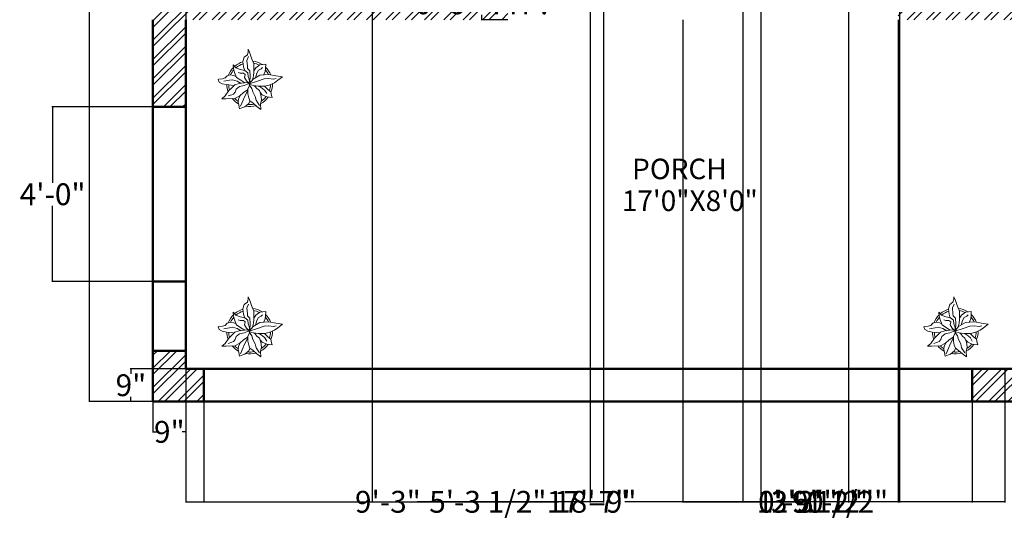
# Model space of a CAD drawing. Units: inches. Extents: x -71 to 434, y -519 to 67.
# Tile 1 of 7: x -49 to 221, y -519 to -377. Entities that reach past the tile are written whole.
import ezdxf

# ---------------------------------------------------------------- set-up
doc = ezdxf.new("R2010")
doc.units = ezdxf.units.IN
doc.header["$MEASUREMENT"] = 0
for name, color, linetype, lineweight in [('A-ANNO-DIMS', 7, 'Continuous', 18), ('A-AREA-IDEN', 7, 'Continuous', 25), ('A-WALL-PATT', 8, 'Continuous', 13), ('CAY', 94, 'Continuous', 13), ('WALL', 50, 'Continuous', 50)]:
    doc.layers.add(name, color=color, linetype=linetype, lineweight=lineweight)
doc.styles.add('ATT', font='romans.shx')
doc.styles.get("Standard").update_dxf_attribs({"font": 'arial.ttf'})
doc.dimstyles.get("Standard").update_dxf_attribs({"dimtxt": 6, "dimasz": 0.18, "dimexe": 0.18, "dimexo": 0.0625, "dimgap": 0.09, "dimtad": 0, "dimtih": 1, "dimtoh": 1, "dimdec": 0, "dimzin": 0, "dimdsep": 46, "dimlunit": 3, "dimtxsty": 'Standard', "dimcen": 0.09, "dimadec": 0, "dimazin": 0, "dimtfac": 1, "dimtdec": 0, "dimtofl": 0, "dimtmove": 0, "dimatfit": 3, "dimfxl": 1, "dimtolj": 1, "dimtzin": 0, "dimarcsym": 0})

# ---------------------------------------------------------------- blocks, each defined once
blk = doc.blocks.new('*D18')
at = {"layer": 'A-ANNO-DIMS', "color": 0, "lineweight": -2, "transparency": 16777216}
for p, q in [((-12.65, 30.83), (-30.15, 30.83)), ((-29.97, 30.65), (-29.97, -222.51)), ((-29.97, -481.99), (-29.97, -228.82)), ((-12.65, -482.17), (-30.15, -482.17))]:
    blk.add_line(p, q, dxfattribs=at)
at = {"layer": 'A-ANNO-DIMS', "color": 0, "transparency": 16777216}
for points in [[(-30, 30.65), (-29.94, 30.65), (-29.97, 30.83)], [(-30, -481.99), (-29.94, -481.99), (-29.97, -482.17)]]:
    blk.add_solid(points, dxfattribs=at)
at = {"layer": 'Defpoints', "color": 0, "transparency": 16777216}
for p in [(-12.59, 30.83), (-29.97, -482.17), (-12.59, -482.17)]:
    blk.add_point(p, dxfattribs=at)
at = {"layer": 'A-ANNO-DIMS', "color": 0, "transparency": 16777216, "insert": (-29.97, -225.67), "char_height": 6, "attachment_point": 5}
blk.add_mtext('\\A1;42\'-9"', dxfattribs=at)
blk = doc.blocks.new('*D19')
at = {"layer": 'A-ANNO-DIMS', "color": 0, "lineweight": -2, "transparency": 16777216}
for p, q in [((-3.65, -473.17), (-18.81, -473.17)), ((-18.63, -473.35), (-18.63, -474.51)), ((-18.63, -481.99), (-18.63, -480.82)), ((-3.65, -482.17), (-18.81, -482.17))]:
    blk.add_line(p, q, dxfattribs=at)
at = {"layer": 'A-ANNO-DIMS', "color": 0, "transparency": 16777216}
for points in [[(-18.66, -473.35), (-18.6, -473.35), (-18.63, -473.17)], [(-18.66, -481.99), (-18.6, -481.99), (-18.63, -482.17)]]:
    blk.add_solid(points, dxfattribs=at)
at = {"layer": 'Defpoints', "color": 0, "transparency": 16777216}
for p in [(-3.59, -473.17), (-18.63, -482.17), (-3.59, -482.17)]:
    blk.add_point(p, dxfattribs=at)
at = {"layer": 'A-ANNO-DIMS', "color": 0, "transparency": 16777216, "insert": (-18.63, -477.67), "char_height": 6, "attachment_point": 5}
blk.add_mtext('\\A1;9"', dxfattribs=at)
blk = doc.blocks.new('*D20')
at = {"layer": 'A-ANNO-DIMS', "color": 0, "lineweight": -2, "transparency": 16777216}
for p, q in [((-12.59, -473.23), (-12.59, -490.67)), ((-3.59, -473.23), (-3.59, -490.67)), ((-12.41, -490.49), (-11.63, -490.49)), ((-3.77, -490.49), (-4.55, -490.49))]:
    blk.add_line(p, q, dxfattribs=at)
at = {"layer": 'A-ANNO-DIMS', "color": 0, "transparency": 16777216}
for points in [[(-12.41, -490.46), (-12.41, -490.52), (-12.59, -490.49)], [(-3.77, -490.46), (-3.77, -490.52), (-3.59, -490.49)]]:
    blk.add_solid(points, dxfattribs=at)
at = {"layer": 'Defpoints', "color": 0, "transparency": 16777216}
for p in [(-12.59, -473.17), (-3.59, -473.17), (-3.59, -490.49)]:
    blk.add_point(p, dxfattribs=at)
at = {"layer": 'A-ANNO-DIMS', "color": 0, "transparency": 16777216, "insert": (-8.09, -490.49), "char_height": 6, "attachment_point": 5}
blk.add_mtext('\\A1;9"', dxfattribs=at)
blk = doc.blocks.new('12PPLT12')
at = {"color": 0, "linetype": 'ByBlock'}
for p, q in [((-0.05, 0.632), (-0.034, 0.694)), ((-0.034, 0.694), (-0.032, 0.751)), ((-0.032, 0.751), (-0.002, 0.689)), ((-0.002, 0.689), (0.044, 0.559)), ((-0.148, 0.486), (-0.116, 0.583)), ((-0.132, 0.367), (-0.148, 0.486)), ((-0.116, 0.583), (-0.05, 0.632)), ((-0.064, 0.51), (-0.026, 0.591)), ((-0.05, 0.38), (-0.064, 0.51)), ((0.044, 0.559), (0.09, 0.432)), ((0.09, 0.432), (0.09, 0.339)), ((-0.349, 0.334), (-0.362, 0.415)), ((-0.362, 0.415), (-0.303, 0.35)), ((-0.332, 0.247), (-0.349, 0.334)), ((-0.289, 0.136), (-0.332, 0.247)), ((-0.303, 0.35), (-0.208, 0.312)), ((-0.205, 0.231), (-0.251, 0.247)), ((-0.208, 0.312), (-0.105, 0.29)), ((-0.137, 0.231), (-0.205, 0.231)), ((-0.097, 0.204), (-0.137, 0.231)), ((-0.108, 0.279), (-0.132, 0.367)), ((-0.105, 0.29), (-0.037, 0.236)), ((-0.043, 0.334), (-0.05, 0.38)), ((0.003, 0.279), (-0.043, 0.334)), ((-0.037, 0.236), (-0.034, 0.158)), ((0.009, 0.169), (0.003, 0.279)), ((0.09, 0.253), (0.082, 0.174)), ((0.09, 0.339), (0.09, 0.253)), ((0.093, 0.282), (0.134, 0.347)), ((0.155, 0.228), (0.131, 0.13)), ((0.134, 0.347), (0.22, 0.415)), ((0.193, 0.293), (0.155, 0.228)), ((0.25, 0.328), (0.193, 0.293)), ((0.22, 0.415), (0.291, 0.421)), ((0.28, 0.353), (0.25, 0.328)), ((0.291, 0.421), (0.35, 0.429)), ((0.342, 0.266), (0.304, 0.19)), ((0.348, 0.331), (0.342, 0.266)), ((0.35, 0.429), (0.348, 0.331)), ((-0.671, 0.098), (-0.687, 0.095)), ((-0.687, 0.095), (-0.666, 0.036)), ((-0.59, 0.109), (-0.671, 0.098)), ((-0.666, 0.036), (-0.601, -0.005)), ((-0.536, 0.125), (-0.59, 0.109)), ((-0.563, 0.052), (-0.441, 0.074)), ((-0.487, 0.171), (-0.536, 0.125)), ((-0.425, 0.193), (-0.487, 0.171)), ((-0.441, 0.074), (-0.373, 0.084)), ((-0.346, 0.179), (-0.425, 0.193)), ((-0.373, 0.084), (-0.27, 0.057)), ((-0.292, 0.149), (-0.346, 0.179)), ((-0.229, 0.003), (-0.324, -0.027)), ((-0.194, 0.074), (-0.289, 0.136)), ((-0.27, 0.057), (-0.186, 0.006)), ((-0.069, 0.027), (-0.229, 0.003)), ((-0.108, 0.019), (-0.194, 0.074)), ((-0.01, 0.003), (-0.121, -0.038)), ((-0.11, 0.133), (-0.097, 0.204)), ((-0.069, 0.06), (-0.11, 0.133)), ((-0.01, 0.014), (-0.069, 0.06)), ((-0.002, 0.006), (-0.069, 0.027)), ((-0.034, 0.158), (-0.007, 0.101)), ((-0.018, -0.008), (0.074, 0.098)), ((-0.01, -0.005), (0.169, 0.055)), ((0.003, 0.017), (-0.01, 0.014)), ((0.003, -0.029), (-0.01, 0.003)), ((-0.007, 0.101), (0.003, 0.017)), ((0.006, 0.027), (0.009, 0.169)), ((0.082, 0.174), (0.061, 0.082)), ((0.074, 0.098), (0.223, 0.188)), ((0.169, 0.055), (0.315, 0.109)), ((0.223, 0.188), (0.421, 0.204)), ((0.315, 0.109), (0.413, 0.117)), ((0.413, 0.117), (0.524, 0.101)), ((0.421, 0.204), (0.573, 0.171)), ((0.545, 0.017), (0.429, -0.032)), ((0.524, 0.101), (0.578, 0.114)), ((0.613, 0.074), (0.545, 0.017)), ((0.573, 0.171), (0.716, 0.152)), ((0.716, 0.152), (0.613, 0.074)), ((-0.601, -0.005), (-0.503, -0.021)), ((-0.452, -0.152), (-0.536, -0.268)), ((-0.503, -0.021), (-0.4, -0.032)), ((-0.395, -0.094), (-0.452, -0.152)), ((-0.4, -0.032), (-0.357, -0.04)), ((-0.324, -0.027), (-0.395, -0.094)), ((-0.316, -0.187), (-0.352, -0.227)), ((-0.292, -0.122), (-0.316, -0.187)), ((-0.224, -0.059), (-0.292, -0.122)), ((-0.121, -0.038), (-0.224, -0.059)), ((-0.213, -0.263), (-0.135, -0.195)), ((-0.135, -0.195), (-0.053, -0.14)), ((-0.119, -0.304), (-0.04, -0.148)), ((-0.053, -0.14), (0.003, -0.029)), ((-0.037, -0.122), (-0.04, -0.219)), ((0.082, -0.038), (-0.018, -0.008)), ((-0.007, -0.024), (0.05, -0.105)), ((0.05, -0.105), (0.071, -0.181)), ((0.071, -0.181), (0.12, -0.282)), ((0.188, -0.054), (0.082, -0.038)), ((0.112, -0.051), (0.09, -0.043)), ((0.155, -0.108), (0.112, -0.051)), ((0.212, -0.152), (0.155, -0.108)), ((0.323, -0.051), (0.188, -0.054)), ((0.247, -0.246), (0.212, -0.152)), ((0.215, -0.062), (0.282, -0.103)), ((0.234, -0.2), (0.277, -0.241)), ((0.282, -0.103), (0.334, -0.146)), ((0.429, -0.032), (0.323, -0.051)), ((0.396, -0.124), (0.326, -0.054)), ((0.334, -0.146), (0.372, -0.217)), ((0.464, -0.176), (0.396, -0.124)), ((0.48, -0.257), (0.464, -0.176)), ((-0.536, -0.268), (-0.606, -0.328)), ((-0.606, -0.328), (-0.522, -0.328)), ((-0.522, -0.328), (-0.324, -0.325)), ((-0.387, -0.241), (-0.465, -0.268)), ((-0.352, -0.227), (-0.387, -0.241)), ((-0.324, -0.325), (-0.213, -0.263)), ((-0.244, -0.33), (-0.247, -0.406)), ((-0.247, -0.406), (-0.233, -0.471)), ((-0.193, -0.236), (-0.244, -0.33)), ((-0.199, -0.494), (-0.139, -0.358)), ((-0.139, -0.358), (-0.119, -0.304)), ((-0.04, -0.219), (-0.021, -0.308)), ((-0.021, -0.308), (0.006, -0.376)), ((-0.017, -0.432), (0.003, -0.378)), ((0.006, -0.376), (0.074, -0.428)), ((0.074, -0.428), (0.158, -0.496)), ((0.12, -0.282), (0.139, -0.363)), ((0.139, -0.363), (0.212, -0.474)), ((0.236, -0.444), (0.261, -0.349)), ((0.261, -0.349), (0.247, -0.246)), ((0.277, -0.241), (0.372, -0.287)), ((0.372, -0.287), (0.494, -0.301)), ((0.494, -0.301), (0.48, -0.257)), ((-0.233, -0.471), (-0.222, -0.551)), ((-0.222, -0.551), (-0.148, -0.522)), ((-0.148, -0.522), (-0.102, -0.503)), ((-0.102, -0.503), (-0.017, -0.432)), ((0.158, -0.496), (0.242, -0.561)), ((0.242, -0.561), (0.236, -0.444))]:
    blk.add_line(p, q, dxfattribs=at)
for radius, start, end in [(0.5, 107.123, 130.9816), (0.458, 107.9864, 130.5771), (0.5, 56.9563, 82.295), (0.458, 62.6899, 79.5345), (0.5, 134.8021, 159.1804), (0.458, 138.4756, 155.3347), (0.458, 26.2761, 41.1349), (0.5, 22.9768, 45.8473), (0.5, 182.503, 200.4563), (0.458, 183.2699, 197.4002), (0.458, 340.6559, 357.5057), (0.5, 338.5862, 359.7442), (0.5, 220.6606, 241.3393), (0.458, 225.0835, 237.5023), (0.5, 298.3455, 324.4541), (0.458, 303.3868, 322.0756), (0.5, 259.7038, 286.1281), (0.458, 264.1886, 282.4028)]:
    blk.add_arc((0, 0), radius, start, end, dxfattribs=at)
at = {"color": 0, "linetype": 'ByBlock', "style": 'ATT'}
for tag, p, flags in [('ITEM', (-1, -3.25), 3), ('ROOM_NUMBER', (-1, -4.583), 1)]:
    blk.add_attdef(tag, p, '', height=1, dxfattribs=dict(at, flags=flags))
blk = doc.blocks.new('*D27')
at = {"layer": 'A-ANNO-DIMS', "color": 0, "lineweight": -2, "transparency": 16777216}
for p, q in [((84.85, -368.17), (77.53, -368.17)), ((77.71, -368.35), (77.71, -369.51)), ((77.71, -376.99), (77.71, -375.82)), ((84.85, -377.17), (77.53, -377.17))]:
    blk.add_line(p, q, dxfattribs=at)
at = {"layer": 'A-ANNO-DIMS', "color": 0, "transparency": 16777216}
for points in [[(77.68, -368.35), (77.74, -368.35), (77.71, -368.17)], [(77.68, -376.99), (77.74, -376.99), (77.71, -377.17)]]:
    blk.add_solid(points, dxfattribs=at)
at = {"layer": 'Defpoints', "color": 0, "transparency": 16777216}
for p in [(77.71, -368.17), (84.91, -368.17), (84.91, -377.17)]:
    blk.add_point(p, dxfattribs=at)
at = {"layer": 'A-ANNO-DIMS', "color": 0, "transparency": 16777216, "insert": (77.71, -372.67), "char_height": 6, "attachment_point": 5}
blk.add_mtext('\\A1;0\'-9" TYP.', dxfattribs=at)
blk = doc.blocks.new('*D47')
at = {"layer": 'A-ANNO-DIMS', "color": 0, "lineweight": -2, "transparency": 16777216}
for p, q in [((132.91, -377.23), (132.91, -509.9)), ((154.41, -377.23), (154.41, -509.9)), ((133.09, -509.72), (154.23, -509.72)), ((154.41, -509.72), (154.59, -509.72))]:
    blk.add_line(p, q, dxfattribs=at)
at = {"layer": 'A-ANNO-DIMS', "color": 0, "transparency": 16777216}
for points in [[(133.09, -509.69), (133.09, -509.75), (132.91, -509.72)], [(154.23, -509.69), (154.23, -509.75), (154.41, -509.72)]]:
    blk.add_solid(points, dxfattribs=at)
at = {"layer": 'Defpoints', "color": 0, "transparency": 16777216}
for p in [(132.91, -377.17), (154.41, -377.17), (154.41, -509.72)]:
    blk.add_point(p, dxfattribs=at)
at = {"layer": 'A-ANNO-DIMS', "color": 0, "transparency": 16777216, "insert": (169.36, -509.72), "char_height": 6, "attachment_point": 5}
blk.add_mtext('\\A1;1\'-9 1/2"', dxfattribs=at)
blk = doc.blocks.new('*D48')
at = {"layer": 'A-ANNO-DIMS', "color": 0, "lineweight": -2, "transparency": 16777216}
for p, q in [((154.41, -377.23), (154.41, -509.9)), ((192.08, -377.23), (192.08, -509.9)), ((154.59, -509.72), (158.19, -509.72)), ((191.9, -509.72), (188.3, -509.72))]:
    blk.add_line(p, q, dxfattribs=at)
at = {"layer": 'A-ANNO-DIMS', "color": 0, "transparency": 16777216}
for points in [[(154.59, -509.69), (154.59, -509.75), (154.41, -509.72)], [(191.9, -509.69), (191.9, -509.75), (192.08, -509.72)]]:
    blk.add_solid(points, dxfattribs=at)
at = {"layer": 'Defpoints', "color": 0, "transparency": 16777216}
for p in [(154.41, -377.17), (192.08, -377.17), (192.08, -509.72)]:
    blk.add_point(p, dxfattribs=at)
at = {"layer": 'A-ANNO-DIMS', "color": 0, "transparency": 16777216, "insert": (173.25, -509.72), "char_height": 6, "attachment_point": 5}
blk.add_mtext('\\A1;3\'-1 1/2"', dxfattribs=at)
blk = doc.blocks.new('*D54')
at = {"layer": 'A-ANNO-DIMS', "color": 0, "lineweight": -2, "transparency": 16777216}
for p, q in [((-3.59, -473.23), (-3.59, -509.9)), ((221.41, -473.23), (221.41, -509.9)), ((-3.41, -509.72), (98.79, -509.72)), ((221.23, -509.72), (119.02, -509.72))]:
    blk.add_line(p, q, dxfattribs=at)
at = {"layer": 'A-ANNO-DIMS', "color": 0, "transparency": 16777216}
for points in [[(-3.41, -509.69), (-3.41, -509.75), (-3.59, -509.72)], [(221.23, -509.69), (221.23, -509.75), (221.41, -509.72)]]:
    blk.add_solid(points, dxfattribs=at)
at = {"layer": 'Defpoints', "color": 0, "transparency": 16777216}
for p in [(-3.59, -473.17), (221.41, -473.17), (221.41, -509.72)]:
    blk.add_point(p, dxfattribs=at)
at = {"layer": 'A-ANNO-DIMS', "color": 0, "transparency": 16777216, "insert": (108.91, -509.72), "char_height": 6, "attachment_point": 5}
blk.add_mtext('\\A1;18\'-9"', dxfattribs=at)
blk = doc.blocks.new('*D56')
at = {"layer": 'A-ANNO-DIMS', "color": 0, "lineweight": -2, "transparency": 16777216}
for p, q in [((154.41, -71.23), (154.41, -509.9)), ((178.41, -71.23), (178.41, -509.9)), ((154.59, -509.72), (158.29, -509.72)), ((178.23, -509.72), (174.52, -509.72))]:
    blk.add_line(p, q, dxfattribs=at)
at = {"layer": 'A-ANNO-DIMS', "color": 0, "transparency": 16777216}
for points in [[(154.59, -509.69), (154.59, -509.75), (154.41, -509.72)], [(178.23, -509.69), (178.23, -509.75), (178.41, -509.72)]]:
    blk.add_solid(points, dxfattribs=at)
at = {"layer": 'Defpoints', "color": 0, "transparency": 16777216}
for p in [(154.41, -71.17), (178.41, -71.17), (178.41, -509.72)]:
    blk.add_point(p, dxfattribs=at)
at = {"layer": 'A-ANNO-DIMS', "color": 0, "transparency": 16777216, "insert": (166.41, -509.72), "char_height": 6, "attachment_point": 5}
blk.add_mtext('\\A1;2\'-0"', dxfattribs=at)
blk = doc.blocks.new('*D62')
at = {"layer": 'A-ANNO-DIMS', "color": 0, "lineweight": -2, "transparency": 16777216}
for p, q in [((149.41, -71.23), (149.41, -509.9)), ((154.41, -71.23), (154.41, -509.9)), ((149.59, -509.72), (154.23, -509.72)), ((154.41, -509.72), (154.59, -509.72))]:
    blk.add_line(p, q, dxfattribs=at)
at = {"layer": 'A-ANNO-DIMS', "color": 0, "transparency": 16777216}
for points in [[(149.59, -509.69), (149.59, -509.75), (149.41, -509.72)], [(154.23, -509.69), (154.23, -509.75), (154.41, -509.72)]]:
    blk.add_solid(points, dxfattribs=at)
at = {"layer": 'Defpoints', "color": 0, "transparency": 16777216}
for p in [(149.41, -71.17), (154.41, -71.17), (154.41, -509.72)]:
    blk.add_point(p, dxfattribs=at)
at = {"layer": 'A-ANNO-DIMS', "color": 0, "transparency": 16777216, "insert": (162.65, -509.72), "char_height": 6, "attachment_point": 5}
blk.add_mtext('\\A1;0\'-5"', dxfattribs=at)
blk = doc.blocks.new('*D66')
at = {"layer": 'A-ANNO-DIMS', "color": 0, "lineweight": -2, "transparency": 16777216}
for p, q in [((-3.59, -119.23), (-3.59, -509.9)), ((107.49, -119.23), (107.49, -509.9)), ((-3.41, -509.72), (43.89, -509.72)), ((107.31, -509.72), (60.02, -509.72))]:
    blk.add_line(p, q, dxfattribs=at)
at = {"layer": 'A-ANNO-DIMS', "color": 0, "transparency": 16777216}
for points in [[(-3.41, -509.69), (-3.41, -509.75), (-3.59, -509.72)], [(107.31, -509.69), (107.31, -509.75), (107.49, -509.72)]]:
    blk.add_solid(points, dxfattribs=at)
at = {"layer": 'Defpoints', "color": 0, "transparency": 16777216}
for p in [(-3.59, -119.17), (107.49, -119.17), (107.49, -509.72)]:
    blk.add_point(p, dxfattribs=at)
at = {"layer": 'A-ANNO-DIMS', "color": 0, "transparency": 16777216, "insert": (51.95, -509.72), "char_height": 6, "attachment_point": 5}
blk.add_mtext('\\A1;9\'-3"', dxfattribs=at)
blk = doc.blocks.new('*D70')
at = {"layer": 'A-ANNO-DIMS', "color": 0, "lineweight": -2, "transparency": 16777216}
for p, q in [((154.41, -224.23), (154.41, -509.9)), ((192.42, -224.23), (192.42, -509.9)), ((154.59, -509.72), (165.35, -509.72)), ((192.24, -509.72), (181.47, -509.72))]:
    blk.add_line(p, q, dxfattribs=at)
at = {"layer": 'A-ANNO-DIMS', "color": 0, "transparency": 16777216}
for points in [[(154.59, -509.69), (154.59, -509.75), (154.41, -509.72)], [(192.24, -509.69), (192.24, -509.75), (192.42, -509.72)]]:
    blk.add_solid(points, dxfattribs=at)
at = {"layer": 'Defpoints', "color": 0, "transparency": 16777216}
for p in [(154.41, -224.17), (192.42, -224.17), (192.42, -509.72)]:
    blk.add_point(p, dxfattribs=at)
at = {"layer": 'A-ANNO-DIMS', "color": 0, "transparency": 16777216, "insert": (173.41, -509.72), "char_height": 6, "attachment_point": 5}
blk.add_mtext('\\A1;3\'-2"', dxfattribs=at)
blk = doc.blocks.new('*D71')
at = {"layer": 'A-ANNO-DIMS', "color": 0, "lineweight": -2, "transparency": 16777216}
for p, q in [((47.64, -300.64), (47.64, -509.9)), ((111.15, -300.64), (111.15, -509.9)), ((47.82, -509.72), (64.34, -509.72)), ((110.97, -509.72), (94.45, -509.72))]:
    blk.add_line(p, q, dxfattribs=at)
at = {"layer": 'A-ANNO-DIMS', "color": 0, "transparency": 16777216}
for points in [[(47.82, -509.69), (47.82, -509.75), (47.64, -509.72)], [(110.97, -509.69), (110.97, -509.75), (111.15, -509.72)]]:
    blk.add_solid(points, dxfattribs=at)
at = {"layer": 'Defpoints', "color": 0, "transparency": 16777216}
for p in [(47.64, -300.57), (111.15, -300.57), (111.15, -509.72)]:
    blk.add_point(p, dxfattribs=at)
at = {"layer": 'A-ANNO-DIMS', "color": 0, "transparency": 16777216, "insert": (79.4, -509.72), "char_height": 6, "attachment_point": 5}
blk.add_mtext('\\A1;5\'-3 1/2"', dxfattribs=at)
blk = doc.blocks.new('*D73')
at = {"layer": 'A-ANNO-DIMS', "color": 0, "lineweight": -2, "transparency": 16777216}
for p, q in [((-12.65, -401.17), (-40.32, -401.17)), ((-40.14, -401.35), (-40.14, -422.01)), ((-40.14, -448.99), (-40.14, -428.32)), ((-12.65, -449.17), (-40.32, -449.17))]:
    blk.add_line(p, q, dxfattribs=at)
at = {"layer": 'A-ANNO-DIMS', "color": 0, "transparency": 16777216}
for points in [[(-40.17, -401.35), (-40.11, -401.35), (-40.14, -401.17)], [(-40.17, -448.99), (-40.11, -448.99), (-40.14, -449.17)]]:
    blk.add_solid(points, dxfattribs=at)
at = {"layer": 'Defpoints', "color": 0, "transparency": 16777216}
for p in [(-12.59, -401.17), (-40.14, -449.17), (-12.59, -449.17)]:
    blk.add_point(p, dxfattribs=at)
at = {"layer": 'A-ANNO-DIMS', "color": 0, "transparency": 16777216, "insert": (-40.14, -425.17), "char_height": 6, "attachment_point": 5}
blk.add_mtext('\\A1;4\'-0"', dxfattribs=at)
blk = doc.blocks.new('*D74')
at = {"layer": 'A-ANNO-DIMS', "color": 0, "lineweight": -2, "transparency": 16777216}
for p, q in [((1.41, -482.23), (1.41, -509.9)), ((212.41, -482.23), (212.41, -509.9)), ((1.59, -509.72), (96.79, -509.72)), ((212.23, -509.72), (117.02, -509.72))]:
    blk.add_line(p, q, dxfattribs=at)
at = {"layer": 'A-ANNO-DIMS', "color": 0, "transparency": 16777216}
for points in [[(1.59, -509.69), (1.59, -509.75), (1.41, -509.72)], [(212.23, -509.69), (212.23, -509.75), (212.41, -509.72)]]:
    blk.add_solid(points, dxfattribs=at)
at = {"layer": 'Defpoints', "color": 0, "transparency": 16777216}
for p in [(1.41, -482.17), (212.41, -482.17), (212.41, -509.72)]:
    blk.add_point(p, dxfattribs=at)
at = {"layer": 'A-ANNO-DIMS', "color": 0, "transparency": 16777216, "insert": (106.91, -509.72), "char_height": 6, "attachment_point": 5}
blk.add_mtext('\\A1;17\'-7"', dxfattribs=at)

msp = doc.modelspace()

# ---------------------------------------------------------------- hatches: boundary and pattern name
at = {"layer": 'A-WALL-PATT'}
h = msp.add_hatch(dxfattribs=at)
h.set_pattern_fill('ANSI32', color=256, scale=10)
h.set_pattern_definition([(45, (-213.138, 0), (-2.65165, 2.65165), []), (45, (-211.37, 0), (-2.65165, 2.65165), [])])
h.paths.add_polyline_path([(383.41, 30.83), (230.41, 30.83), (149.41, 30.83), (-12.59, 30.83), (-12.59, -20.17), (-3.59, -20.17), (-3.59, 21.83), (140.41, 21.83), (140.41, 15.83), (149.41, 15.83), (149.41, 21.83), (221.41, 21.83), (221.41, 15.83), (230.41, 15.83), (230.41, 21.83), (374.41, 21.83), (374.41, -110.17), (369.41, -110.17), (369.41, -119.17), (374.41, -119.17), (374.41, -215.17), (320.41, -215.17), (320.41, -119.17), (345.41, -119.17), (345.41, -110.17), (221.41, -110.17), (221.41, -119.17), (311.41, -119.17), (311.41, -215.17), (192.42, -215.17), (192.42, -224.17), (221.41, -224.17), (221.41, -228.23), (230.41, -228.23), (230.41, -224.17), (374.41, -224.17), (374.41, -368.17), (230.41, -368.17), (230.41, -266.34), (221.41, -266.34), (221.41, -368.17), (192.08, -368.17), (192.08, -377.17), (230.41, -377.17), (374.41, -377.17), (374.41, -473.17), (230.41, -473.17), (212.41, -473.17), (212.41, -482.17), (383.41, -482.17), (383.41, -377.17), (383.41, -224.17), (383.41, -119.17)])
h.paths.add_polyline_path([(149.41, -110.17), (-3.59, -110.17), (-3.59, -68.17), (-12.59, -68.17), (-12.59, -276.67), (-3.59, -276.67), (-3.59, -224.17), (154.41, -224.17), (154.41, -215.17), (149.41, -215.17), (149.41, -154.17), (140.41, -154.17), (140.41, -215.17), (-3.59, -215.17), (-3.59, -119.17), (19.82, -119.17), (140.41, -119.17), (140.41, -124.17), (149.41, -124.17)])
h.paths.add_polyline_path([(84.91, -368.17), (-3.59, -368.17), (-3.59, -324.67), (-12.59, -324.67), (-12.59, -377.17), (-12.59, -401.17), (-3.59, -401.17), (-3.59, -377.17), (84.91, -377.17)], flags=17)
h.paths.add_polyline_path([(1.41, -473.17), (-3.59, -473.17), (-3.59, -468.17), (-12.59, -468.17), (-12.59, -482.17), (1.41, -482.17)], flags=17)

# ---------------------------------------------------------------- linework, layer by layer
at = {"layer": 'WALL'}
for p, q in [((-12.59, -377.17), (-12.59, -401.17)), ((-3.59, -377.17), (-3.59, -401.17)), ((-12.59, -401.17), (-3.59, -401.17)), ((-12.59, -401.17), (-12.59, -449.17)), ((-3.59, -401.17), (-3.59, -449.17)), ((-12.59, -449.17), (-12.59, -482.17)), ((-12.59, -449.17), (-3.59, -449.17)), ((-3.59, -449.17), (-3.59, -473.17)), ((-12.59, -468.17), (-3.59, -468.17)), ((-3.59, -473.17), (230.41, -473.17)), ((1.41, -473.17), (1.41, -482.17)), ((212.41, -473.17), (212.41, -482.17)), ((-12.59, -482.17), (383.41, -482.17))]:
    msp.add_line(p, q, dxfattribs=at)

# ---------------------------------------------------------------- block references
at = {"layer": 'CAY', "xscale": 12.58515090877727, "yscale": 12.58515090877727, "zscale": 12.58515090877727}
for p in [(13.97, -394.77), (13.97, -462.78), (207.77, -462.78)]:
    msp.add_blockref('12PPLT12', p, dxfattribs=at)

# ---------------------------------------------------------------- texts
at = {"layer": 'A-AREA-IDEN'}
for s, p in [('PORCH', (119.01, -421.02)), ('17\'0"X8\'0"', (116.18, -429.77))]:
    msp.add_text(s, height=5.643, dxfattribs=at).set_placement(p)

# ---------------------------------------------------------------- dimensions: what is measured, and where the dimension line sits
at = {"layer": 'A-ANNO-DIMS'}
for base, p1, p2, override, picture, middle in [((-29.97, -482.17), (-12.59, 30.83), (-12.59, -482.17), {"dimclrd": 0, "dimclre": 0, "dimclrt": 0}, '*D18', (-29.97, -225.67)), ((-40.14, -449.17), (-12.59, -401.17), (-12.59, -449.17), {"dimdec": 1, "dimlfac": 1, "dimrnd": 0, "dimzin": 1, "dimdsep": 46, "dimlunit": 4, "dimfrac": 2}, '*D73', (-40.14, -425.17)), ((-18.63, -482.17), (-3.59, -473.17), (-3.59, -482.17), {"dimclrd": 0, "dimclre": 0, "dimclrt": 0}, '*D19', (-18.63, -477.67))]:
    dim = msp.add_linear_dim(base=base, p1=p1, p2=p2, angle=90, dimstyle='Standard', override=override, dxfattribs=at)
    dim.commit()
    dim.dimension.update_dxf_attribs({"geometry": picture, "text_midpoint": middle})
for base, p1, p2, override, picture, middle in [((154.41, -509.72), (149.41, -71.17), (154.41, -71.17), {"dimdec": 1, "dimlfac": 1, "dimrnd": 0, "dimzin": 1, "dimdsep": 46, "dimlunit": 4, "dimfrac": 2}, '*D62', (162.65, -509.72)), ((178.41, -509.72), (154.41, -71.17), (178.41, -71.17), {"dimdec": 1, "dimlfac": 1, "dimrnd": 0, "dimzin": 1, "dimdsep": 46, "dimlunit": 4, "dimfrac": 2}, '*D56', (166.41, -509.72)), ((107.49, -509.72), (-3.59, -119.17), (107.49, -119.17), {"dimdec": 1, "dimlfac": 1, "dimrnd": 0, "dimzin": 1, "dimdsep": 46, "dimlunit": 4, "dimfrac": 2}, '*D66', (51.95, -509.72)), ((192.42, -509.72), (154.41, -224.17), (192.42, -224.17), {"dimdec": 1, "dimlfac": 1, "dimrnd": 0, "dimzin": 1, "dimdsep": 46, "dimlunit": 4, "dimfrac": 2}, '*D70', (173.41, -509.72)), ((111.15, -509.72), (47.64, -300.57), (111.15, -300.57), {"dimdec": 1, "dimlfac": 1, "dimrnd": 0, "dimzin": 1, "dimdsep": 46, "dimlunit": 4, "dimfrac": 2}, '*D71', (79.4, -509.72)), ((154.41, -509.72), (132.91, -377.17), (154.41, -377.17), {"dimdec": 1, "dimlfac": 1, "dimrnd": 0, "dimzin": 1, "dimdsep": 46, "dimlunit": 4, "dimfrac": 2}, '*D47', (169.36, -509.72)), ((192.08, -509.72), (154.41, -377.17), (192.08, -377.17), {"dimdec": 1, "dimlfac": 1, "dimrnd": 0, "dimzin": 1, "dimdsep": 46, "dimlunit": 4, "dimfrac": 2}, '*D48', (173.25, -509.72)), ((-3.59, -490.49), (-12.59, -473.17), (-3.59, -473.17), {"dimclrd": 0, "dimclre": 0, "dimclrt": 0}, '*D20', (-8.09, -490.49)), ((221.41, -509.72), (-3.59, -473.17), (221.41, -473.17), {"dimdec": 1, "dimlfac": 1, "dimrnd": 0, "dimzin": 1, "dimdsep": 46, "dimlunit": 4, "dimfrac": 2}, '*D54', (108.91, -509.72)), ((212.41, -509.72), (1.41, -482.17), (212.41, -482.17), {"dimdec": 1, "dimlfac": 1, "dimrnd": 0, "dimzin": 1, "dimdsep": 46, "dimlunit": 4, "dimfrac": 2}, '*D74', (106.91, -509.72))]:
    dim = msp.add_linear_dim(base=base, p1=p1, p2=p2, dimstyle='Standard', override=override, dxfattribs=at)
    dim.commit()
    dim.dimension.update_dxf_attribs({"geometry": picture, "text_midpoint": middle})
dim = msp.add_linear_dim(base=(77.71, -368.17), p1=(84.91, -377.17), p2=(84.91, -368.17), angle=90, text='<> TYP.', dimstyle='Standard', override={"dimdec": 1, "dimlfac": 1, "dimrnd": 0, "dimzin": 1, "dimdsep": 46, "dimlunit": 4, "dimfrac": 2}, dxfattribs=at)
dim.commit()
dim.dimension.update_dxf_attribs({"geometry": '*D27', "text_midpoint": (77.71, -372.67)})

doc.saveas('drawing.dxf')
